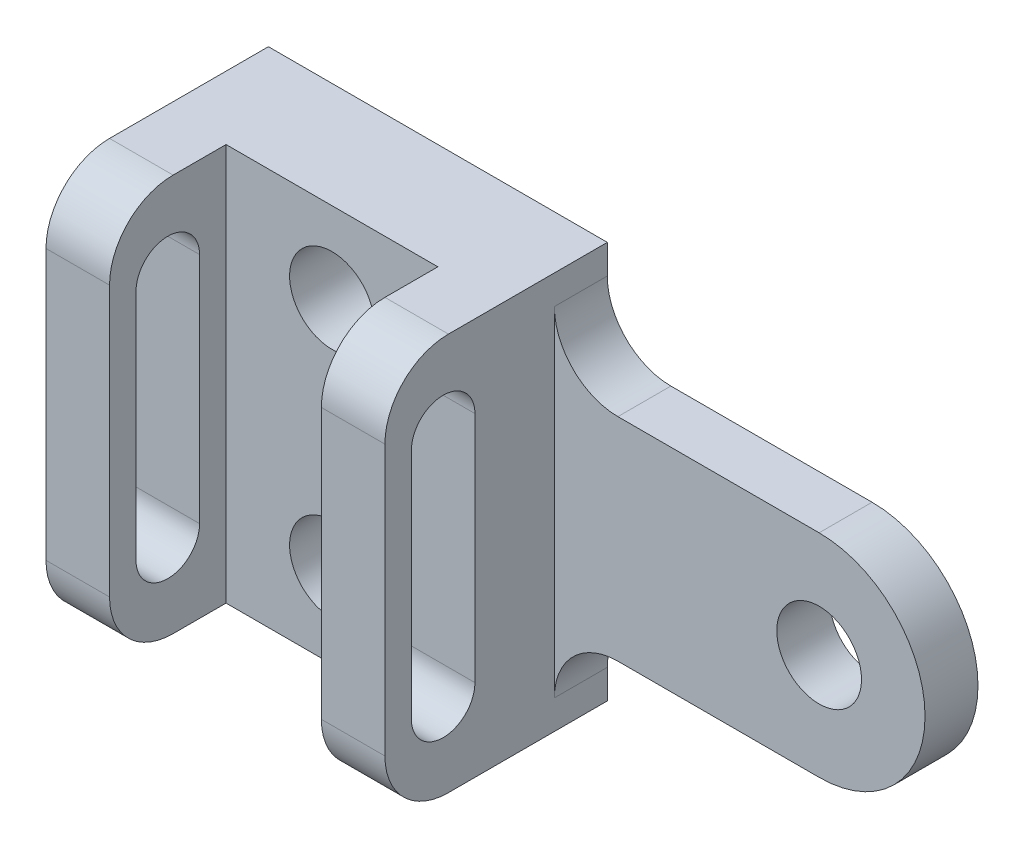
ISO-10303-21;
HEADER;
FILE_DESCRIPTION(('STEP AP214'),'2;1');
FILE_NAME('part.step','',(''),(''),'','','');
FILE_SCHEMA(('AUTOMOTIVE_DESIGN { 1 0 10303 214 1 1 1 1 }'));
ENDSEC;
DATA;
#1=APPLICATION_CONTEXT('core data for automotive mechanical design processes');
#2=APPLICATION_PROTOCOL_DEFINITION('international standard','automotive_design',2000,#1);
#3=PRODUCT_CONTEXT('',#1,'mechanical');
#4=PRODUCT('Part','Part','',(#3));
#5=PRODUCT_RELATED_PRODUCT_CATEGORY('part','',(#4));
#6=PRODUCT_DEFINITION_FORMATION('','',#4);
#7=PRODUCT_DEFINITION_CONTEXT('part definition',#1,'design');
#8=PRODUCT_DEFINITION('design','',#6,#7);
#9=PRODUCT_DEFINITION_SHAPE('','',#8);
#10=(LENGTH_UNIT() NAMED_UNIT(*) SI_UNIT(.MILLI.,.METRE.));
#11=(NAMED_UNIT(*) PLANE_ANGLE_UNIT() SI_UNIT($,.RADIAN.));
#12=(NAMED_UNIT(*) SI_UNIT($,.STERADIAN.) SOLID_ANGLE_UNIT());
#13=UNCERTAINTY_MEASURE_WITH_UNIT(LENGTH_MEASURE(1.E-05),#10,'distance_accuracy_value','');
#14=(GEOMETRIC_REPRESENTATION_CONTEXT(3) GLOBAL_UNCERTAINTY_ASSIGNED_CONTEXT((#13)) GLOBAL_UNIT_ASSIGNED_CONTEXT((#10,
#11,#12)) REPRESENTATION_CONTEXT('',''));
#15=CARTESIAN_POINT('',(0.,0.,0.));
#16=DIRECTION('',(0.,0.,1.));
#17=DIRECTION('',(1.,0.,0.));
#18=AXIS2_PLACEMENT_3D('',#15,#16,#17);
#19=CARTESIAN_POINT('',(0.,0.,20.));
#20=DIRECTION('',(0.,0.,1.));
#21=DIRECTION('',(1.,0.,0.));
#22=AXIS2_PLACEMENT_3D('',#19,#20,#21);
#23=PLANE('',#22);
#24=CARTESIAN_POINT('',(32.,59.5,20.));
#25=DIRECTION('',(0.,0.,1.));
#26=DIRECTION('',(1.,0.,0.));
#27=AXIS2_PLACEMENT_3D('',#24,#25,#26);
#28=CIRCLE('',#27,8.);
#29=CARTESIAN_POINT('',(40.,59.5,20.));
#30=VERTEX_POINT('',#29);
#31=EDGE_CURVE('E454',#30,#30,#28,.T.);
#32=ORIENTED_EDGE('',*,*,#31,.F.);
#33=EDGE_LOOP('',(#32));
#34=FACE_BOUND('',#33,.T.);
#35=CARTESIAN_POINT('',(32.,15.5,20.));
#36=DIRECTION('',(0.,0.,1.));
#37=DIRECTION('',(1.,0.,0.));
#38=AXIS2_PLACEMENT_3D('',#35,#36,#37);
#39=CIRCLE('',#38,8.);
#40=CARTESIAN_POINT('',(40.,15.5,20.));
#41=VERTEX_POINT('',#40);
#42=EDGE_CURVE('E450',#41,#41,#39,.T.);
#43=ORIENTED_EDGE('',*,*,#42,.F.);
#44=EDGE_LOOP('',(#43));
#45=FACE_BOUND('',#44,.T.);
#46=DIRECTION('',(1.,0.,0.));
#47=VECTOR('',#46,1.);
#48=CARTESIAN_POINT('',(0.,0.,20.));
#49=LINE('',#48,#47);
#50=CARTESIAN_POINT('',(12.,0.,20.));
#51=VERTEX_POINT('',#50);
#52=CARTESIAN_POINT('',(52.,0.,20.));
#53=VERTEX_POINT('',#52);
#54=EDGE_CURVE('E334',#51,#53,#49,.T.);
#55=ORIENTED_EDGE('',*,*,#54,.T.);
#56=DIRECTION('',(0.,-1.,0.));
#57=VECTOR('',#56,1.);
#58=CARTESIAN_POINT('',(52.,75.,20.));
#59=LINE('',#58,#57);
#60=CARTESIAN_POINT('',(52.,75.,20.));
#61=VERTEX_POINT('',#60);
#62=EDGE_CURVE('E305',#61,#53,#59,.T.);
#63=ORIENTED_EDGE('',*,*,#62,.F.);
#64=DIRECTION('',(-1.,0.,0.));
#65=VECTOR('',#64,1.);
#66=CARTESIAN_POINT('',(64.,75.,20.));
#67=LINE('',#66,#65);
#68=CARTESIAN_POINT('',(12.,75.,20.));
#69=VERTEX_POINT('',#68);
#70=EDGE_CURVE('E336',#61,#69,#67,.T.);
#71=ORIENTED_EDGE('',*,*,#70,.T.);
#72=DIRECTION('',(0.,1.,0.));
#73=VECTOR('',#72,1.);
#74=CARTESIAN_POINT('',(12.,75.,20.));
#75=LINE('',#74,#73);
#76=EDGE_CURVE('E322',#51,#69,#75,.T.);
#77=ORIENTED_EDGE('',*,*,#76,.F.);
#78=EDGE_LOOP('',(#55,#63,#71,#77));
#79=FACE_BOUND('',#78,.T.);
#80=ADVANCED_FACE('F39',(#34,#45,#79),#23,.T.);
#81=CARTESIAN_POINT('',(0.,75.,20.));
#82=DIRECTION('',(1.,0.,0.));
#83=DIRECTION('',(0.,0.,-1.));
#84=AXIS2_PLACEMENT_3D('',#81,#82,#83);
#85=PLANE('',#84);
#86=DIRECTION('',(0.,-1.,0.));
#87=VECTOR('',#86,1.);
#88=CARTESIAN_POINT('',(0.,15.5,37.));
#89=LINE('',#88,#87);
#90=CARTESIAN_POINT('',(0.,59.5,37.));
#91=VERTEX_POINT('',#90);
#92=CARTESIAN_POINT('',(0.,15.5,37.));
#93=VERTEX_POINT('',#92);
#94=EDGE_CURVE('E290',#91,#93,#89,.T.);
#95=ORIENTED_EDGE('',*,*,#94,.T.);
#96=CARTESIAN_POINT('',(0.,15.5,31.));
#97=DIRECTION('',(1.,0.,0.));
#98=DIRECTION('',(0.,1.,0.));
#99=AXIS2_PLACEMENT_3D('',#96,#97,#98);
#100=CIRCLE('',#99,6.00000000000001);
#101=CARTESIAN_POINT('',(0.,15.5,25.));
#102=VERTEX_POINT('',#101);
#103=EDGE_CURVE('E280',#93,#102,#100,.T.);
#104=ORIENTED_EDGE('',*,*,#103,.T.);
#105=DIRECTION('',(0.,1.,0.));
#106=VECTOR('',#105,1.);
#107=CARTESIAN_POINT('',(0.,15.5,25.));
#108=LINE('',#107,#106);
#109=CARTESIAN_POINT('',(0.,59.5,25.));
#110=VERTEX_POINT('',#109);
#111=EDGE_CURVE('E278',#102,#110,#108,.T.);
#112=ORIENTED_EDGE('',*,*,#111,.T.);
#113=CARTESIAN_POINT('',(0.,59.5,31.));
#114=DIRECTION('',(1.,0.,0.));
#115=DIRECTION('',(0.,1.,0.));
#116=AXIS2_PLACEMENT_3D('',#113,#114,#115);
#117=CIRCLE('',#116,6.00000000000001);
#118=EDGE_CURVE('E283',#110,#91,#117,.T.);
#119=ORIENTED_EDGE('',*,*,#118,.T.);
#120=EDGE_LOOP('',(#95,#104,#112,#119));
#121=FACE_BOUND('',#120,.T.);
#122=DIRECTION('',(0.,0.,-1.));
#123=VECTOR('',#122,1.);
#124=CARTESIAN_POINT('',(0.,0.,20.));
#125=LINE('',#124,#123);
#126=CARTESIAN_POINT('',(0.,0.,30.));
#127=VERTEX_POINT('',#126);
#128=CARTESIAN_POINT('',(0.,0.,0.));
#129=VERTEX_POINT('',#128);
#130=EDGE_CURVE('E356',#127,#129,#125,.T.);
#131=ORIENTED_EDGE('',*,*,#130,.F.);
#132=CARTESIAN_POINT('',(0.,12.,30.));
#133=DIRECTION('',(1.,0.,0.));
#134=DIRECTION('',(0.,0.,-1.));
#135=AXIS2_PLACEMENT_3D('',#132,#133,#134);
#136=CIRCLE('',#135,12.);
#137=CARTESIAN_POINT('',(0.,12.,42.));
#138=VERTEX_POINT('',#137);
#139=EDGE_CURVE('E372',#127,#138,#136,.F.);
#140=ORIENTED_EDGE('',*,*,#139,.T.);
#141=DIRECTION('',(0.,-1.,0.));
#142=VECTOR('',#141,1.);
#143=CARTESIAN_POINT('',(0.,75.,42.));
#144=LINE('',#143,#142);
#145=CARTESIAN_POINT('',(0.,63.,42.));
#146=VERTEX_POINT('',#145);
#147=EDGE_CURVE('E325',#146,#138,#144,.T.);
#148=ORIENTED_EDGE('',*,*,#147,.F.);
#149=CARTESIAN_POINT('',(0.,63.,30.));
#150=DIRECTION('',(1.,0.,0.));
#151=DIRECTION('',(0.,0.,-1.));
#152=AXIS2_PLACEMENT_3D('',#149,#150,#151);
#153=CIRCLE('',#152,12.);
#154=CARTESIAN_POINT('',(0.,75.,30.));
#155=VERTEX_POINT('',#154);
#156=EDGE_CURVE('E375',#146,#155,#153,.F.);
#157=ORIENTED_EDGE('',*,*,#156,.T.);
#158=DIRECTION('',(0.,0.,-1.));
#159=VECTOR('',#158,1.);
#160=CARTESIAN_POINT('',(0.,75.,20.));
#161=LINE('',#160,#159);
#162=CARTESIAN_POINT('',(0.,75.,0.));
#163=VERTEX_POINT('',#162);
#164=EDGE_CURVE('E345',#155,#163,#161,.T.);
#165=ORIENTED_EDGE('',*,*,#164,.T.);
#166=DIRECTION('',(0.,-1.,0.));
#167=VECTOR('',#166,1.);
#168=CARTESIAN_POINT('',(0.,75.,0.));
#169=LINE('',#168,#167);
#170=EDGE_CURVE('E332',#163,#129,#169,.T.);
#171=ORIENTED_EDGE('',*,*,#170,.T.);
#172=EDGE_LOOP('',(#131,#140,#148,#157,#165,#171));
#173=FACE_BOUND('',#172,.T.);
#174=ADVANCED_FACE('F472',(#121,#173),#85,.F.);
#175=CARTESIAN_POINT('',(0.,0.,20.));
#176=DIRECTION('',(0.,1.,0.));
#177=DIRECTION('',(0.,0.,1.));
#178=AXIS2_PLACEMENT_3D('',#175,#176,#177);
#179=PLANE('',#178);
#180=DIRECTION('',(0.,0.,-1.));
#181=VECTOR('',#180,1.);
#182=CARTESIAN_POINT('',(64.,0.,20.));
#183=LINE('',#182,#181);
#184=CARTESIAN_POINT('',(64.,0.,30.));
#185=VERTEX_POINT('',#184);
#186=CARTESIAN_POINT('',(64.,0.,0.));
#187=VERTEX_POINT('',#186);
#188=EDGE_CURVE('E358',#185,#187,#183,.T.);
#189=ORIENTED_EDGE('',*,*,#188,.F.);
#190=DIRECTION('',(1.,0.,0.));
#191=VECTOR('',#190,1.);
#192=CARTESIAN_POINT('',(52.,0.,30.));
#193=LINE('',#192,#191);
#194=CARTESIAN_POINT('',(52.,0.,30.));
#195=VERTEX_POINT('',#194);
#196=EDGE_CURVE('E65',#185,#195,#193,.F.);
#197=ORIENTED_EDGE('',*,*,#196,.T.);
#198=DIRECTION('',(0.,0.,-1.));
#199=VECTOR('',#198,1.);
#200=CARTESIAN_POINT('',(52.,0.,42.));
#201=LINE('',#200,#199);
#202=EDGE_CURVE('E316',#195,#53,#201,.T.);
#203=ORIENTED_EDGE('',*,*,#202,.T.);
#204=ORIENTED_EDGE('',*,*,#54,.F.);
#205=DIRECTION('',(0.,0.,-1.));
#206=VECTOR('',#205,1.);
#207=CARTESIAN_POINT('',(12.,0.,42.));
#208=LINE('',#207,#206);
#209=CARTESIAN_POINT('',(12.,0.,30.));
#210=VERTEX_POINT('',#209);
#211=EDGE_CURVE('E335',#210,#51,#208,.T.);
#212=ORIENTED_EDGE('',*,*,#211,.F.);
#213=DIRECTION('',(1.,0.,0.));
#214=VECTOR('',#213,1.);
#215=CARTESIAN_POINT('',(0.,0.,30.));
#216=LINE('',#215,#214);
#217=EDGE_CURVE('E369',#210,#127,#216,.F.);
#218=ORIENTED_EDGE('',*,*,#217,.T.);
#219=ORIENTED_EDGE('',*,*,#130,.T.);
#220=DIRECTION('',(1.,0.,0.));
#221=VECTOR('',#220,1.);
#222=CARTESIAN_POINT('',(0.,0.,0.));
#223=LINE('',#222,#221);
#224=EDGE_CURVE('E343',#129,#187,#223,.T.);
#225=ORIENTED_EDGE('',*,*,#224,.T.);
#226=EDGE_LOOP('',(#189,#197,#203,#204,#212,#218,#219,#225));
#227=FACE_BOUND('',#226,.T.);
#228=ADVANCED_FACE('F399',(#227),#179,.F.);
#229=CARTESIAN_POINT('',(64.,0.,20.));
#230=DIRECTION('',(-1.,0.,0.));
#231=DIRECTION('',(0.,0.,1.));
#232=AXIS2_PLACEMENT_3D('',#229,#230,#231);
#233=PLANE('',#232);
#234=DIRECTION('',(0.,-1.,0.));
#235=VECTOR('',#234,1.);
#236=CARTESIAN_POINT('',(64.,15.5,25.));
#237=LINE('',#236,#235);
#238=CARTESIAN_POINT('',(64.,59.5,25.));
#239=VERTEX_POINT('',#238);
#240=CARTESIAN_POINT('',(64.,15.5,25.));
#241=VERTEX_POINT('',#240);
#242=EDGE_CURVE('E260',#239,#241,#237,.T.);
#243=ORIENTED_EDGE('',*,*,#242,.T.);
#244=CARTESIAN_POINT('',(64.,15.5,31.));
#245=DIRECTION('',(-1.,0.,0.));
#246=DIRECTION('',(0.,-1.,0.));
#247=AXIS2_PLACEMENT_3D('',#244,#245,#246);
#248=CIRCLE('',#247,6.);
#249=CARTESIAN_POINT('',(64.,15.5,37.));
#250=VERTEX_POINT('',#249);
#251=EDGE_CURVE('E250',#241,#250,#248,.T.);
#252=ORIENTED_EDGE('',*,*,#251,.T.);
#253=DIRECTION('',(0.,1.,0.));
#254=VECTOR('',#253,1.);
#255=CARTESIAN_POINT('',(64.,15.5,37.));
#256=LINE('',#255,#254);
#257=CARTESIAN_POINT('',(64.,59.5,37.));
#258=VERTEX_POINT('',#257);
#259=EDGE_CURVE('E249',#250,#258,#256,.T.);
#260=ORIENTED_EDGE('',*,*,#259,.T.);
#261=CARTESIAN_POINT('',(64.,59.5,31.));
#262=DIRECTION('',(-1.,0.,0.));
#263=DIRECTION('',(0.,-1.,0.));
#264=AXIS2_PLACEMENT_3D('',#261,#262,#263);
#265=CIRCLE('',#264,6.);
#266=EDGE_CURVE('E251',#258,#239,#265,.T.);
#267=ORIENTED_EDGE('',*,*,#266,.T.);
#268=EDGE_LOOP('',(#243,#252,#260,#267));
#269=FACE_BOUND('',#268,.T.);
#270=DIRECTION('',(0.,1.,0.));
#271=VECTOR('',#270,1.);
#272=CARTESIAN_POINT('',(64.,75.,42.));
#273=LINE('',#272,#271);
#274=CARTESIAN_POINT('',(64.,12.,42.));
#275=VERTEX_POINT('',#274);
#276=CARTESIAN_POINT('',(64.,63.,42.));
#277=VERTEX_POINT('',#276);
#278=EDGE_CURVE('E315',#275,#277,#273,.T.);
#279=ORIENTED_EDGE('',*,*,#278,.F.);
#280=CARTESIAN_POINT('',(64.,12.,30.));
#281=DIRECTION('',(-1.,0.,0.));
#282=DIRECTION('',(0.,0.,1.));
#283=AXIS2_PLACEMENT_3D('',#280,#281,#282);
#284=CIRCLE('',#283,12.);
#285=EDGE_CURVE('E387',#275,#185,#284,.F.);
#286=ORIENTED_EDGE('',*,*,#285,.T.);
#287=ORIENTED_EDGE('',*,*,#188,.T.);
#288=DIRECTION('',(0.,1.,0.));
#289=VECTOR('',#288,1.);
#290=CARTESIAN_POINT('',(64.,0.,0.));
#291=LINE('',#290,#289);
#292=CARTESIAN_POINT('',(64.,5.49999999999997,0.));
#293=VERTEX_POINT('',#292);
#294=EDGE_CURVE('E348',#187,#293,#291,.T.);
#295=ORIENTED_EDGE('',*,*,#294,.T.);
#296=DIRECTION('',(0.,0.,-1.));
#297=VECTOR('',#296,1.);
#298=CARTESIAN_POINT('',(64.,5.49999999999997,10.));
#299=LINE('',#298,#297);
#300=CARTESIAN_POINT('',(64.,5.49999999999997,10.));
#301=VERTEX_POINT('',#300);
#302=EDGE_CURVE('E411',#301,#293,#299,.T.);
#303=ORIENTED_EDGE('',*,*,#302,.F.);
#304=DIRECTION('',(0.,-1.,0.));
#305=VECTOR('',#304,1.);
#306=CARTESIAN_POINT('',(64.,69.5,10.));
#307=LINE('',#306,#305);
#308=CARTESIAN_POINT('',(64.,69.5,10.));
#309=VERTEX_POINT('',#308);
#310=EDGE_CURVE('E438',#309,#301,#307,.T.);
#311=ORIENTED_EDGE('',*,*,#310,.F.);
#312=DIRECTION('',(0.,0.,-1.));
#313=VECTOR('',#312,1.);
#314=CARTESIAN_POINT('',(64.,69.5,10.));
#315=LINE('',#314,#313);
#316=CARTESIAN_POINT('',(64.,69.5,0.));
#317=VERTEX_POINT('',#316);
#318=EDGE_CURVE('E243',#309,#317,#315,.T.);
#319=ORIENTED_EDGE('',*,*,#318,.T.);
#320=CARTESIAN_POINT('',(64.,75.,0.));
#321=VERTEX_POINT('',#320);
#322=EDGE_CURVE('E350',#317,#321,#291,.T.);
#323=ORIENTED_EDGE('',*,*,#322,.T.);
#324=DIRECTION('',(0.,0.,-1.));
#325=VECTOR('',#324,1.);
#326=CARTESIAN_POINT('',(64.,75.,20.));
#327=LINE('',#326,#325);
#328=CARTESIAN_POINT('',(64.,75.,30.));
#329=VERTEX_POINT('',#328);
#330=EDGE_CURVE('E352',#329,#321,#327,.T.);
#331=ORIENTED_EDGE('',*,*,#330,.F.);
#332=CARTESIAN_POINT('',(64.,63.,30.));
#333=DIRECTION('',(-1.,0.,0.));
#334=DIRECTION('',(0.,0.,1.));
#335=AXIS2_PLACEMENT_3D('',#332,#333,#334);
#336=CIRCLE('',#335,12.);
#337=EDGE_CURVE('E381',#329,#277,#336,.F.);
#338=ORIENTED_EDGE('',*,*,#337,.T.);
#339=EDGE_LOOP('',(#279,#286,#287,#295,#303,#311,#319,#323,#331,#338));
#340=FACE_BOUND('',#339,.T.);
#341=ADVANCED_FACE('F397',(#269,#340),#233,.F.);
#342=CARTESIAN_POINT('',(64.,75.,20.));
#343=DIRECTION('',(0.,-1.,0.));
#344=DIRECTION('',(0.,0.,-1.));
#345=AXIS2_PLACEMENT_3D('',#342,#343,#344);
#346=PLANE('',#345);
#347=DIRECTION('',(0.,0.,-1.));
#348=VECTOR('',#347,1.);
#349=CARTESIAN_POINT('',(52.,75.,42.));
#350=LINE('',#349,#348);
#351=CARTESIAN_POINT('',(52.,75.,30.));
#352=VERTEX_POINT('',#351);
#353=EDGE_CURVE('E314',#352,#61,#350,.T.);
#354=ORIENTED_EDGE('',*,*,#353,.F.);
#355=DIRECTION('',(-1.,0.,0.));
#356=VECTOR('',#355,1.);
#357=CARTESIAN_POINT('',(64.,75.,30.));
#358=LINE('',#357,#356);
#359=EDGE_CURVE('E11',#352,#329,#358,.F.);
#360=ORIENTED_EDGE('',*,*,#359,.T.);
#361=ORIENTED_EDGE('',*,*,#330,.T.);
#362=DIRECTION('',(-1.,0.,0.));
#363=VECTOR('',#362,1.);
#364=CARTESIAN_POINT('',(64.,75.,0.));
#365=LINE('',#364,#363);
#366=EDGE_CURVE('E339',#321,#163,#365,.T.);
#367=ORIENTED_EDGE('',*,*,#366,.T.);
#368=ORIENTED_EDGE('',*,*,#164,.F.);
#369=DIRECTION('',(-1.,0.,0.));
#370=VECTOR('',#369,1.);
#371=CARTESIAN_POINT('',(12.,75.,30.));
#372=LINE('',#371,#370);
#373=CARTESIAN_POINT('',(12.,75.,30.));
#374=VERTEX_POINT('',#373);
#375=EDGE_CURVE('E376',#155,#374,#372,.F.);
#376=ORIENTED_EDGE('',*,*,#375,.T.);
#377=DIRECTION('',(0.,0.,-1.));
#378=VECTOR('',#377,1.);
#379=CARTESIAN_POINT('',(12.,75.,42.));
#380=LINE('',#379,#378);
#381=EDGE_CURVE('E330',#374,#69,#380,.T.);
#382=ORIENTED_EDGE('',*,*,#381,.T.);
#383=ORIENTED_EDGE('',*,*,#70,.F.);
#384=EDGE_LOOP('',(#354,#360,#361,#367,#368,#376,#382,#383));
#385=FACE_BOUND('',#384,.T.);
#386=ADVANCED_FACE('F485',(#385),#346,.F.);
#387=CARTESIAN_POINT('',(0.,0.,0.));
#388=DIRECTION('',(0.,0.,1.));
#389=DIRECTION('',(1.,0.,0.));
#390=AXIS2_PLACEMENT_3D('',#387,#388,#389);
#391=PLANE('',#390);
#392=CARTESIAN_POINT('',(32.,59.5,0.));
#393=DIRECTION('',(0.,0.,1.));
#394=DIRECTION('',(1.,0.,0.));
#395=AXIS2_PLACEMENT_3D('',#392,#393,#394);
#396=CIRCLE('',#395,8.);
#397=CARTESIAN_POINT('',(40.,59.5,0.));
#398=VERTEX_POINT('',#397);
#399=EDGE_CURVE('E443',#398,#398,#396,.T.);
#400=ORIENTED_EDGE('',*,*,#399,.T.);
#401=EDGE_LOOP('',(#400));
#402=FACE_BOUND('',#401,.T.);
#403=CARTESIAN_POINT('',(32.,15.5,0.));
#404=DIRECTION('',(0.,0.,1.));
#405=DIRECTION('',(1.,0.,0.));
#406=AXIS2_PLACEMENT_3D('',#403,#404,#405);
#407=CIRCLE('',#406,8.);
#408=CARTESIAN_POINT('',(40.,15.5,0.));
#409=VERTEX_POINT('',#408);
#410=EDGE_CURVE('E448',#409,#409,#407,.T.);
#411=ORIENTED_EDGE('',*,*,#410,.T.);
#412=EDGE_LOOP('',(#411));
#413=FACE_BOUND('',#412,.T.);
#414=ORIENTED_EDGE('',*,*,#170,.F.);
#415=ORIENTED_EDGE('',*,*,#366,.F.);
#416=ORIENTED_EDGE('',*,*,#322,.F.);
#417=CARTESIAN_POINT('',(76.,69.5,0.));
#418=DIRECTION('',(0.,0.,-1.));
#419=DIRECTION('',(1.,0.,0.));
#420=AXIS2_PLACEMENT_3D('',#417,#418,#419);
#421=CIRCLE('',#420,12.);
#422=CARTESIAN_POINT('',(76.,57.5,0.));
#423=VERTEX_POINT('',#422);
#424=EDGE_CURVE('E429',#423,#317,#421,.T.);
#425=ORIENTED_EDGE('',*,*,#424,.F.);
#426=DIRECTION('',(-1.,0.,0.));
#427=VECTOR('',#426,1.);
#428=CARTESIAN_POINT('',(114.,57.5,0.));
#429=LINE('',#428,#427);
#430=CARTESIAN_POINT('',(114.,57.5,0.));
#431=VERTEX_POINT('',#430);
#432=EDGE_CURVE('E435',#431,#423,#429,.T.);
#433=ORIENTED_EDGE('',*,*,#432,.F.);
#434=CARTESIAN_POINT('',(114.,37.5,0.));
#435=DIRECTION('',(0.,0.,1.));
#436=DIRECTION('',(1.,0.,0.));
#437=AXIS2_PLACEMENT_3D('',#434,#435,#436);
#438=CIRCLE('',#437,20.);
#439=CARTESIAN_POINT('',(114.,17.5,0.));
#440=VERTEX_POINT('',#439);
#441=EDGE_CURVE('E238',#440,#431,#438,.T.);
#442=ORIENTED_EDGE('',*,*,#441,.F.);
#443=DIRECTION('',(1.,0.,0.));
#444=VECTOR('',#443,1.);
#445=CARTESIAN_POINT('',(114.,17.5,0.));
#446=LINE('',#445,#444);
#447=CARTESIAN_POINT('',(76.,17.5,0.));
#448=VERTEX_POINT('',#447);
#449=EDGE_CURVE('E234',#448,#440,#446,.T.);
#450=ORIENTED_EDGE('',*,*,#449,.F.);
#451=CARTESIAN_POINT('',(76.,5.49999999999997,0.));
#452=DIRECTION('',(0.,0.,-1.));
#453=DIRECTION('',(1.,0.,0.));
#454=AXIS2_PLACEMENT_3D('',#451,#452,#453);
#455=CIRCLE('',#454,12.);
#456=EDGE_CURVE('E408',#293,#448,#455,.T.);
#457=ORIENTED_EDGE('',*,*,#456,.F.);
#458=ORIENTED_EDGE('',*,*,#294,.F.);
#459=ORIENTED_EDGE('',*,*,#224,.F.);
#460=EDGE_LOOP('',(#414,#415,#416,#425,#433,#442,#450,#457,#458,#459));
#461=FACE_BOUND('',#460,.T.);
#462=CARTESIAN_POINT('',(114.,37.5,0.));
#463=DIRECTION('',(0.,0.,1.));
#464=DIRECTION('',(1.,0.,0.));
#465=AXIS2_PLACEMENT_3D('',#462,#463,#464);
#466=CIRCLE('',#465,8.);
#467=CARTESIAN_POINT('',(122.,37.5,0.));
#468=VERTEX_POINT('',#467);
#469=EDGE_CURVE('E441',#468,#468,#466,.T.);
#470=ORIENTED_EDGE('',*,*,#469,.T.);
#471=EDGE_LOOP('',(#470));
#472=FACE_BOUND('',#471,.T.);
#473=ADVANCED_FACE('F410',(#402,#413,#461,#472),#391,.F.);
#474=CARTESIAN_POINT('',(12.,75.,42.));
#475=DIRECTION('',(-1.,0.,0.));
#476=DIRECTION('',(0.,-1.,0.));
#477=AXIS2_PLACEMENT_3D('',#474,#475,#476);
#478=PLANE('',#477);
#479=DIRECTION('',(0.,1.,0.));
#480=VECTOR('',#479,1.);
#481=CARTESIAN_POINT('',(12.,15.5,25.));
#482=LINE('',#481,#480);
#483=CARTESIAN_POINT('',(12.,15.5,25.));
#484=VERTEX_POINT('',#483);
#485=CARTESIAN_POINT('',(12.,59.5,25.));
#486=VERTEX_POINT('',#485);
#487=EDGE_CURVE('E292',#484,#486,#482,.T.);
#488=ORIENTED_EDGE('',*,*,#487,.F.);
#489=CARTESIAN_POINT('',(12.,15.5,31.));
#490=DIRECTION('',(1.,0.,0.));
#491=DIRECTION('',(0.,1.,0.));
#492=AXIS2_PLACEMENT_3D('',#489,#490,#491);
#493=CIRCLE('',#492,6.00000000000001);
#494=CARTESIAN_POINT('',(12.,15.5,37.));
#495=VERTEX_POINT('',#494);
#496=EDGE_CURVE('E269',#495,#484,#493,.T.);
#497=ORIENTED_EDGE('',*,*,#496,.F.);
#498=DIRECTION('',(0.,-1.,0.));
#499=VECTOR('',#498,1.);
#500=CARTESIAN_POINT('',(12.,15.5,37.));
#501=LINE('',#500,#499);
#502=CARTESIAN_POINT('',(12.,59.5,37.));
#503=VERTEX_POINT('',#502);
#504=EDGE_CURVE('E284',#503,#495,#501,.T.);
#505=ORIENTED_EDGE('',*,*,#504,.F.);
#506=CARTESIAN_POINT('',(12.,59.5,31.));
#507=DIRECTION('',(1.,0.,0.));
#508=DIRECTION('',(0.,1.,0.));
#509=AXIS2_PLACEMENT_3D('',#506,#507,#508);
#510=CIRCLE('',#509,6.00000000000001);
#511=EDGE_CURVE('E294',#486,#503,#510,.T.);
#512=ORIENTED_EDGE('',*,*,#511,.F.);
#513=EDGE_LOOP('',(#488,#497,#505,#512));
#514=FACE_BOUND('',#513,.T.);
#515=DIRECTION('',(0.,1.,0.));
#516=VECTOR('',#515,1.);
#517=CARTESIAN_POINT('',(12.,75.,42.));
#518=LINE('',#517,#516);
#519=CARTESIAN_POINT('',(12.,12.,42.));
#520=VERTEX_POINT('',#519);
#521=CARTESIAN_POINT('',(12.,63.,42.));
#522=VERTEX_POINT('',#521);
#523=EDGE_CURVE('E323',#520,#522,#518,.T.);
#524=ORIENTED_EDGE('',*,*,#523,.F.);
#525=CARTESIAN_POINT('',(12.,12.,30.));
#526=DIRECTION('',(-1.,0.,0.));
#527=DIRECTION('',(0.,-1.,0.));
#528=AXIS2_PLACEMENT_3D('',#525,#526,#527);
#529=CIRCLE('',#528,12.);
#530=EDGE_CURVE('E368',#520,#210,#529,.F.);
#531=ORIENTED_EDGE('',*,*,#530,.T.);
#532=ORIENTED_EDGE('',*,*,#211,.T.);
#533=ORIENTED_EDGE('',*,*,#76,.T.);
#534=ORIENTED_EDGE('',*,*,#381,.F.);
#535=CARTESIAN_POINT('',(12.,63.,30.));
#536=DIRECTION('',(-1.,0.,0.));
#537=DIRECTION('',(0.,-1.,0.));
#538=AXIS2_PLACEMENT_3D('',#535,#536,#537);
#539=CIRCLE('',#538,12.);
#540=EDGE_CURVE('E366',#374,#522,#539,.F.);
#541=ORIENTED_EDGE('',*,*,#540,.T.);
#542=EDGE_LOOP('',(#524,#531,#532,#533,#534,#541));
#543=FACE_BOUND('',#542,.T.);
#544=ADVANCED_FACE('F488',(#514,#543),#478,.F.);
#545=CARTESIAN_POINT('',(0.,0.,42.));
#546=DIRECTION('',(0.,0.,1.));
#547=DIRECTION('',(1.,0.,0.));
#548=AXIS2_PLACEMENT_3D('',#545,#546,#547);
#549=PLANE('',#548);
#550=ORIENTED_EDGE('',*,*,#147,.T.);
#551=DIRECTION('',(1.,0.,0.));
#552=VECTOR('',#551,1.);
#553=CARTESIAN_POINT('',(12.,12.,42.));
#554=LINE('',#553,#552);
#555=EDGE_CURVE('E361',#138,#520,#554,.T.);
#556=ORIENTED_EDGE('',*,*,#555,.T.);
#557=ORIENTED_EDGE('',*,*,#523,.T.);
#558=DIRECTION('',(-1.,0.,0.));
#559=VECTOR('',#558,1.);
#560=CARTESIAN_POINT('',(0.,63.,42.));
#561=LINE('',#560,#559);
#562=EDGE_CURVE('E359',#522,#146,#561,.T.);
#563=ORIENTED_EDGE('',*,*,#562,.T.);
#564=EDGE_LOOP('',(#550,#556,#557,#563));
#565=FACE_BOUND('',#564,.T.);
#566=ADVANCED_FACE('F492',(#565),#549,.T.);
#567=CARTESIAN_POINT('',(52.,75.,42.));
#568=DIRECTION('',(1.,0.,0.));
#569=DIRECTION('',(0.,1.,0.));
#570=AXIS2_PLACEMENT_3D('',#567,#568,#569);
#571=PLANE('',#570);
#572=DIRECTION('',(0.,1.,0.));
#573=VECTOR('',#572,1.);
#574=CARTESIAN_POINT('',(52.,15.5,37.));
#575=LINE('',#574,#573);
#576=CARTESIAN_POINT('',(52.,15.5,37.));
#577=VERTEX_POINT('',#576);
#578=CARTESIAN_POINT('',(52.,59.5,37.));
#579=VERTEX_POINT('',#578);
#580=EDGE_CURVE('E241',#577,#579,#575,.T.);
#581=ORIENTED_EDGE('',*,*,#580,.F.);
#582=CARTESIAN_POINT('',(52.,15.5,31.));
#583=DIRECTION('',(-1.,0.,0.));
#584=DIRECTION('',(0.,-1.,0.));
#585=AXIS2_PLACEMENT_3D('',#582,#583,#584);
#586=CIRCLE('',#585,6.);
#587=CARTESIAN_POINT('',(52.,15.5,25.));
#588=VERTEX_POINT('',#587);
#589=EDGE_CURVE('E237',#588,#577,#586,.T.);
#590=ORIENTED_EDGE('',*,*,#589,.F.);
#591=DIRECTION('',(0.,-1.,0.));
#592=VECTOR('',#591,1.);
#593=CARTESIAN_POINT('',(52.,15.5,25.));
#594=LINE('',#593,#592);
#595=CARTESIAN_POINT('',(52.,59.5,25.));
#596=VERTEX_POINT('',#595);
#597=EDGE_CURVE('E252',#596,#588,#594,.T.);
#598=ORIENTED_EDGE('',*,*,#597,.F.);
#599=CARTESIAN_POINT('',(52.,59.5,31.));
#600=DIRECTION('',(-1.,0.,0.));
#601=DIRECTION('',(0.,-1.,0.));
#602=AXIS2_PLACEMENT_3D('',#599,#600,#601);
#603=CIRCLE('',#602,6.);
#604=EDGE_CURVE('E265',#579,#596,#603,.T.);
#605=ORIENTED_EDGE('',*,*,#604,.F.);
#606=EDGE_LOOP('',(#581,#590,#598,#605));
#607=FACE_BOUND('',#606,.T.);
#608=ORIENTED_EDGE('',*,*,#202,.F.);
#609=CARTESIAN_POINT('',(52.,12.,30.));
#610=DIRECTION('',(1.,0.,0.));
#611=DIRECTION('',(0.,1.,0.));
#612=AXIS2_PLACEMENT_3D('',#609,#610,#611);
#613=CIRCLE('',#612,12.);
#614=CARTESIAN_POINT('',(52.,12.,42.));
#615=VERTEX_POINT('',#614);
#616=EDGE_CURVE('E50',#195,#615,#613,.F.);
#617=ORIENTED_EDGE('',*,*,#616,.T.);
#618=DIRECTION('',(0.,-1.,0.));
#619=VECTOR('',#618,1.);
#620=CARTESIAN_POINT('',(52.,75.,42.));
#621=LINE('',#620,#619);
#622=CARTESIAN_POINT('',(52.,63.,42.));
#623=VERTEX_POINT('',#622);
#624=EDGE_CURVE('E307',#623,#615,#621,.T.);
#625=ORIENTED_EDGE('',*,*,#624,.F.);
#626=CARTESIAN_POINT('',(52.,63.,30.));
#627=DIRECTION('',(1.,0.,0.));
#628=DIRECTION('',(0.,1.,0.));
#629=AXIS2_PLACEMENT_3D('',#626,#627,#628);
#630=CIRCLE('',#629,12.);
#631=EDGE_CURVE('E53',#623,#352,#630,.F.);
#632=ORIENTED_EDGE('',*,*,#631,.T.);
#633=ORIENTED_EDGE('',*,*,#353,.T.);
#634=ORIENTED_EDGE('',*,*,#62,.T.);
#635=EDGE_LOOP('',(#608,#617,#625,#632,#633,#634));
#636=FACE_BOUND('',#635,.T.);
#637=ADVANCED_FACE('F388',(#607,#636),#571,.F.);
#638=CARTESIAN_POINT('',(0.,0.,42.));
#639=DIRECTION('',(0.,0.,1.));
#640=DIRECTION('',(1.,0.,0.));
#641=AXIS2_PLACEMENT_3D('',#638,#639,#640);
#642=PLANE('',#641);
#643=ORIENTED_EDGE('',*,*,#624,.T.);
#644=DIRECTION('',(1.,0.,0.));
#645=VECTOR('',#644,1.);
#646=CARTESIAN_POINT('',(64.,12.,42.));
#647=LINE('',#646,#645);
#648=EDGE_CURVE('E382',#615,#275,#647,.T.);
#649=ORIENTED_EDGE('',*,*,#648,.T.);
#650=ORIENTED_EDGE('',*,*,#278,.T.);
#651=DIRECTION('',(-1.,0.,0.));
#652=VECTOR('',#651,1.);
#653=CARTESIAN_POINT('',(52.,63.,42.));
#654=LINE('',#653,#652);
#655=EDGE_CURVE('E377',#277,#623,#654,.T.);
#656=ORIENTED_EDGE('',*,*,#655,.T.);
#657=EDGE_LOOP('',(#643,#649,#650,#656));
#658=FACE_BOUND('',#657,.T.);
#659=ADVANCED_FACE('F393',(#658),#642,.T.);
#660=CARTESIAN_POINT('',(0.,15.5,31.));
#661=DIRECTION('',(1.,0.,0.));
#662=DIRECTION('',(0.,1.,0.));
#663=AXIS2_PLACEMENT_3D('',#660,#661,#662);
#664=CYLINDRICAL_SURFACE('',#663,6.00000000000001);
#665=ORIENTED_EDGE('',*,*,#496,.T.);
#666=DIRECTION('',(1.,0.,0.));
#667=VECTOR('',#666,1.);
#668=CARTESIAN_POINT('',(0.,15.5,25.));
#669=LINE('',#668,#667);
#670=EDGE_CURVE('E289',#102,#484,#669,.T.);
#671=ORIENTED_EDGE('',*,*,#670,.F.);
#672=ORIENTED_EDGE('',*,*,#103,.F.);
#673=DIRECTION('',(1.,0.,0.));
#674=VECTOR('',#673,1.);
#675=CARTESIAN_POINT('',(0.,15.5,37.));
#676=LINE('',#675,#674);
#677=EDGE_CURVE('E297',#93,#495,#676,.T.);
#678=ORIENTED_EDGE('',*,*,#677,.T.);
#679=EDGE_LOOP('',(#665,#671,#672,#678));
#680=FACE_BOUND('',#679,.T.);
#681=ADVANCED_FACE('F547',(#680),#664,.F.);
#682=CARTESIAN_POINT('',(0.,15.5,37.));
#683=DIRECTION('',(0.,0.,1.));
#684=DIRECTION('',(1.,0.,0.));
#685=AXIS2_PLACEMENT_3D('',#682,#683,#684);
#686=PLANE('',#685);
#687=ORIENTED_EDGE('',*,*,#504,.T.);
#688=ORIENTED_EDGE('',*,*,#677,.F.);
#689=ORIENTED_EDGE('',*,*,#94,.F.);
#690=DIRECTION('',(1.,0.,0.));
#691=VECTOR('',#690,1.);
#692=CARTESIAN_POINT('',(0.,59.5,37.));
#693=LINE('',#692,#691);
#694=EDGE_CURVE('E303',#91,#503,#693,.T.);
#695=ORIENTED_EDGE('',*,*,#694,.T.);
#696=EDGE_LOOP('',(#687,#688,#689,#695));
#697=FACE_BOUND('',#696,.T.);
#698=ADVANCED_FACE('F542',(#697),#686,.F.);
#699=CARTESIAN_POINT('',(0.,59.5,31.));
#700=DIRECTION('',(1.,0.,0.));
#701=DIRECTION('',(0.,1.,0.));
#702=AXIS2_PLACEMENT_3D('',#699,#700,#701);
#703=CYLINDRICAL_SURFACE('',#702,6.00000000000001);
#704=ORIENTED_EDGE('',*,*,#511,.T.);
#705=ORIENTED_EDGE('',*,*,#694,.F.);
#706=ORIENTED_EDGE('',*,*,#118,.F.);
#707=DIRECTION('',(1.,0.,0.));
#708=VECTOR('',#707,1.);
#709=CARTESIAN_POINT('',(0.,59.5,25.));
#710=LINE('',#709,#708);
#711=EDGE_CURVE('E304',#110,#486,#710,.T.);
#712=ORIENTED_EDGE('',*,*,#711,.T.);
#713=EDGE_LOOP('',(#704,#705,#706,#712));
#714=FACE_BOUND('',#713,.T.);
#715=ADVANCED_FACE('F548',(#714),#703,.F.);
#716=CARTESIAN_POINT('',(0.,15.5,25.));
#717=DIRECTION('',(0.,0.,-1.));
#718=DIRECTION('',(-1.,0.,0.));
#719=AXIS2_PLACEMENT_3D('',#716,#717,#718);
#720=PLANE('',#719);
#721=ORIENTED_EDGE('',*,*,#487,.T.);
#722=ORIENTED_EDGE('',*,*,#711,.F.);
#723=ORIENTED_EDGE('',*,*,#111,.F.);
#724=ORIENTED_EDGE('',*,*,#670,.T.);
#725=EDGE_LOOP('',(#721,#722,#723,#724));
#726=FACE_BOUND('',#725,.T.);
#727=ADVANCED_FACE('F545',(#726),#720,.F.);
#728=CARTESIAN_POINT('',(64.,15.5,31.));
#729=DIRECTION('',(-1.,0.,0.));
#730=DIRECTION('',(0.,-1.,0.));
#731=AXIS2_PLACEMENT_3D('',#728,#729,#730);
#732=CYLINDRICAL_SURFACE('',#731,6.);
#733=ORIENTED_EDGE('',*,*,#589,.T.);
#734=DIRECTION('',(-1.,0.,0.));
#735=VECTOR('',#734,1.);
#736=CARTESIAN_POINT('',(64.,15.5,37.));
#737=LINE('',#736,#735);
#738=EDGE_CURVE('E256',#250,#577,#737,.T.);
#739=ORIENTED_EDGE('',*,*,#738,.F.);
#740=ORIENTED_EDGE('',*,*,#251,.F.);
#741=DIRECTION('',(-1.,0.,0.));
#742=VECTOR('',#741,1.);
#743=CARTESIAN_POINT('',(64.,15.5,25.));
#744=LINE('',#743,#742);
#745=EDGE_CURVE('E268',#241,#588,#744,.T.);
#746=ORIENTED_EDGE('',*,*,#745,.T.);
#747=EDGE_LOOP('',(#733,#739,#740,#746));
#748=FACE_BOUND('',#747,.T.);
#749=ADVANCED_FACE('F535',(#748),#732,.F.);
#750=CARTESIAN_POINT('',(64.,15.5,25.));
#751=DIRECTION('',(0.,0.,-1.));
#752=DIRECTION('',(-1.,0.,0.));
#753=AXIS2_PLACEMENT_3D('',#750,#751,#752);
#754=PLANE('',#753);
#755=ORIENTED_EDGE('',*,*,#597,.T.);
#756=ORIENTED_EDGE('',*,*,#745,.F.);
#757=ORIENTED_EDGE('',*,*,#242,.F.);
#758=DIRECTION('',(-1.,0.,0.));
#759=VECTOR('',#758,1.);
#760=CARTESIAN_POINT('',(64.,59.5,25.));
#761=LINE('',#760,#759);
#762=EDGE_CURVE('E272',#239,#596,#761,.T.);
#763=ORIENTED_EDGE('',*,*,#762,.T.);
#764=EDGE_LOOP('',(#755,#756,#757,#763));
#765=FACE_BOUND('',#764,.T.);
#766=ADVANCED_FACE('F528',(#765),#754,.F.);
#767=CARTESIAN_POINT('',(64.,59.5,31.));
#768=DIRECTION('',(-1.,0.,0.));
#769=DIRECTION('',(0.,-1.,0.));
#770=AXIS2_PLACEMENT_3D('',#767,#768,#769);
#771=CYLINDRICAL_SURFACE('',#770,6.);
#772=ORIENTED_EDGE('',*,*,#604,.T.);
#773=ORIENTED_EDGE('',*,*,#762,.F.);
#774=ORIENTED_EDGE('',*,*,#266,.F.);
#775=DIRECTION('',(-1.,0.,0.));
#776=VECTOR('',#775,1.);
#777=CARTESIAN_POINT('',(64.,59.5,37.));
#778=LINE('',#777,#776);
#779=EDGE_CURVE('E271',#258,#579,#778,.T.);
#780=ORIENTED_EDGE('',*,*,#779,.T.);
#781=EDGE_LOOP('',(#772,#773,#774,#780));
#782=FACE_BOUND('',#781,.T.);
#783=ADVANCED_FACE('F532',(#782),#771,.F.);
#784=CARTESIAN_POINT('',(64.,15.5,37.));
#785=DIRECTION('',(0.,0.,1.));
#786=DIRECTION('',(1.,0.,0.));
#787=AXIS2_PLACEMENT_3D('',#784,#785,#786);
#788=PLANE('',#787);
#789=ORIENTED_EDGE('',*,*,#580,.T.);
#790=ORIENTED_EDGE('',*,*,#779,.F.);
#791=ORIENTED_EDGE('',*,*,#259,.F.);
#792=ORIENTED_EDGE('',*,*,#738,.T.);
#793=EDGE_LOOP('',(#789,#790,#791,#792));
#794=FACE_BOUND('',#793,.T.);
#795=ADVANCED_FACE('F537',(#794),#788,.F.);
#796=CARTESIAN_POINT('',(114.,37.5,10.));
#797=DIRECTION('',(0.,0.,1.));
#798=DIRECTION('',(1.,0.,0.));
#799=AXIS2_PLACEMENT_3D('',#796,#797,#798);
#800=PLANE('',#799);
#801=CARTESIAN_POINT('',(114.,37.5,10.));
#802=DIRECTION('',(0.,0.,1.));
#803=DIRECTION('',(1.,0.,0.));
#804=AXIS2_PLACEMENT_3D('',#801,#802,#803);
#805=CIRCLE('',#804,20.);
#806=CARTESIAN_POINT('',(114.,17.5,10.));
#807=VERTEX_POINT('',#806);
#808=CARTESIAN_POINT('',(114.,57.5,10.));
#809=VERTEX_POINT('',#808);
#810=EDGE_CURVE('E222',#807,#809,#805,.T.);
#811=ORIENTED_EDGE('',*,*,#810,.T.);
#812=DIRECTION('',(-1.,0.,0.));
#813=VECTOR('',#812,1.);
#814=CARTESIAN_POINT('',(114.,57.5,10.));
#815=LINE('',#814,#813);
#816=CARTESIAN_POINT('',(76.,57.5,10.));
#817=VERTEX_POINT('',#816);
#818=EDGE_CURVE('E215',#809,#817,#815,.T.);
#819=ORIENTED_EDGE('',*,*,#818,.T.);
#820=CARTESIAN_POINT('',(76.,69.5,10.));
#821=DIRECTION('',(0.,0.,-1.));
#822=DIRECTION('',(1.,0.,0.));
#823=AXIS2_PLACEMENT_3D('',#820,#821,#822);
#824=CIRCLE('',#823,12.);
#825=EDGE_CURVE('E223',#817,#309,#824,.T.);
#826=ORIENTED_EDGE('',*,*,#825,.T.);
#827=ORIENTED_EDGE('',*,*,#310,.T.);
#828=CARTESIAN_POINT('',(76.,5.49999999999997,10.));
#829=DIRECTION('',(0.,0.,-1.));
#830=DIRECTION('',(1.,0.,0.));
#831=AXIS2_PLACEMENT_3D('',#828,#829,#830);
#832=CIRCLE('',#831,12.);
#833=CARTESIAN_POINT('',(76.,17.5,10.));
#834=VERTEX_POINT('',#833);
#835=EDGE_CURVE('E417',#301,#834,#832,.T.);
#836=ORIENTED_EDGE('',*,*,#835,.T.);
#837=DIRECTION('',(1.,0.,0.));
#838=VECTOR('',#837,1.);
#839=CARTESIAN_POINT('',(114.,17.5,10.));
#840=LINE('',#839,#838);
#841=EDGE_CURVE('E229',#834,#807,#840,.T.);
#842=ORIENTED_EDGE('',*,*,#841,.T.);
#843=EDGE_LOOP('',(#811,#819,#826,#827,#836,#842));
#844=FACE_BOUND('',#843,.T.);
#845=CARTESIAN_POINT('',(114.,37.5,10.));
#846=DIRECTION('',(0.,0.,1.));
#847=DIRECTION('',(1.,0.,0.));
#848=AXIS2_PLACEMENT_3D('',#845,#846,#847);
#849=CIRCLE('',#848,8.);
#850=CARTESIAN_POINT('',(122.,37.5,10.));
#851=VERTEX_POINT('',#850);
#852=EDGE_CURVE('E434',#851,#851,#849,.T.);
#853=ORIENTED_EDGE('',*,*,#852,.F.);
#854=EDGE_LOOP('',(#853));
#855=FACE_BOUND('',#854,.T.);
#856=ADVANCED_FACE('F227',(#844,#855),#800,.T.);
#857=CARTESIAN_POINT('',(114.,37.5,10.));
#858=DIRECTION('',(0.,0.,-1.));
#859=DIRECTION('',(-1.,0.,0.));
#860=AXIS2_PLACEMENT_3D('',#857,#858,#859);
#861=CYLINDRICAL_SURFACE('',#860,20.);
#862=ORIENTED_EDGE('',*,*,#441,.T.);
#863=DIRECTION('',(0.,0.,-1.));
#864=VECTOR('',#863,1.);
#865=CARTESIAN_POINT('',(114.,57.5,10.));
#866=LINE('',#865,#864);
#867=EDGE_CURVE('E219',#809,#431,#866,.T.);
#868=ORIENTED_EDGE('',*,*,#867,.F.);
#869=ORIENTED_EDGE('',*,*,#810,.F.);
#870=DIRECTION('',(0.,0.,-1.));
#871=VECTOR('',#870,1.);
#872=CARTESIAN_POINT('',(114.,17.5,10.));
#873=LINE('',#872,#871);
#874=EDGE_CURVE('E421',#807,#440,#873,.T.);
#875=ORIENTED_EDGE('',*,*,#874,.T.);
#876=EDGE_LOOP('',(#862,#868,#869,#875));
#877=FACE_BOUND('',#876,.T.);
#878=ADVANCED_FACE('F236',(#877),#861,.T.);
#879=CARTESIAN_POINT('',(114.,57.5,10.));
#880=DIRECTION('',(0.,-1.,0.));
#881=DIRECTION('',(0.,0.,-1.));
#882=AXIS2_PLACEMENT_3D('',#879,#880,#881);
#883=PLANE('',#882);
#884=ORIENTED_EDGE('',*,*,#432,.T.);
#885=DIRECTION('',(0.,0.,-1.));
#886=VECTOR('',#885,1.);
#887=CARTESIAN_POINT('',(76.,57.5,10.));
#888=LINE('',#887,#886);
#889=EDGE_CURVE('E218',#817,#423,#888,.T.);
#890=ORIENTED_EDGE('',*,*,#889,.F.);
#891=ORIENTED_EDGE('',*,*,#818,.F.);
#892=ORIENTED_EDGE('',*,*,#867,.T.);
#893=EDGE_LOOP('',(#884,#890,#891,#892));
#894=FACE_BOUND('',#893,.T.);
#895=ADVANCED_FACE('F211',(#894),#883,.F.);
#896=CARTESIAN_POINT('',(76.,69.5,10.));
#897=DIRECTION('',(0.,0.,-1.));
#898=DIRECTION('',(-1.,0.,0.));
#899=AXIS2_PLACEMENT_3D('',#896,#897,#898);
#900=CYLINDRICAL_SURFACE('',#899,12.);
#901=ORIENTED_EDGE('',*,*,#424,.T.);
#902=ORIENTED_EDGE('',*,*,#318,.F.);
#903=ORIENTED_EDGE('',*,*,#825,.F.);
#904=ORIENTED_EDGE('',*,*,#889,.T.);
#905=EDGE_LOOP('',(#901,#902,#903,#904));
#906=FACE_BOUND('',#905,.T.);
#907=ADVANCED_FACE('F510',(#906),#900,.F.);
#908=CARTESIAN_POINT('',(76.,5.49999999999997,10.));
#909=DIRECTION('',(0.,0.,-1.));
#910=DIRECTION('',(-1.,0.,0.));
#911=AXIS2_PLACEMENT_3D('',#908,#909,#910);
#912=CYLINDRICAL_SURFACE('',#911,12.);
#913=ORIENTED_EDGE('',*,*,#456,.T.);
#914=DIRECTION('',(0.,0.,-1.));
#915=VECTOR('',#914,1.);
#916=CARTESIAN_POINT('',(76.,17.5,10.));
#917=LINE('',#916,#915);
#918=EDGE_CURVE('E419',#834,#448,#917,.T.);
#919=ORIENTED_EDGE('',*,*,#918,.F.);
#920=ORIENTED_EDGE('',*,*,#835,.F.);
#921=ORIENTED_EDGE('',*,*,#302,.T.);
#922=EDGE_LOOP('',(#913,#919,#920,#921));
#923=FACE_BOUND('',#922,.T.);
#924=ADVANCED_FACE('F416',(#923),#912,.F.);
#925=CARTESIAN_POINT('',(114.,17.5,10.));
#926=DIRECTION('',(0.,1.,0.));
#927=DIRECTION('',(0.,0.,1.));
#928=AXIS2_PLACEMENT_3D('',#925,#926,#927);
#929=PLANE('',#928);
#930=ORIENTED_EDGE('',*,*,#449,.T.);
#931=ORIENTED_EDGE('',*,*,#874,.F.);
#932=ORIENTED_EDGE('',*,*,#841,.F.);
#933=ORIENTED_EDGE('',*,*,#918,.T.);
#934=EDGE_LOOP('',(#930,#931,#932,#933));
#935=FACE_BOUND('',#934,.T.);
#936=ADVANCED_FACE('F508',(#935),#929,.F.);
#937=CARTESIAN_POINT('',(114.,37.5,10.));
#938=DIRECTION('',(0.,0.,-1.));
#939=DIRECTION('',(-1.,0.,0.));
#940=AXIS2_PLACEMENT_3D('',#937,#938,#939);
#941=CYLINDRICAL_SURFACE('',#940,8.);
#942=ORIENTED_EDGE('',*,*,#852,.T.);
#943=EDGE_LOOP('',(#942));
#944=FACE_BOUND('',#943,.T.);
#945=ORIENTED_EDGE('',*,*,#469,.F.);
#946=EDGE_LOOP('',(#945));
#947=FACE_BOUND('',#946,.T.);
#948=ADVANCED_FACE('F512',(#944,#947),#941,.F.);
#949=CARTESIAN_POINT('',(32.,15.5,0.));
#950=DIRECTION('',(0.,0.,1.));
#951=DIRECTION('',(1.,0.,0.));
#952=AXIS2_PLACEMENT_3D('',#949,#950,#951);
#953=CYLINDRICAL_SURFACE('',#952,8.);
#954=ORIENTED_EDGE('',*,*,#410,.F.);
#955=EDGE_LOOP('',(#954));
#956=FACE_BOUND('',#955,.T.);
#957=ORIENTED_EDGE('',*,*,#42,.T.);
#958=EDGE_LOOP('',(#957));
#959=FACE_BOUND('',#958,.T.);
#960=ADVANCED_FACE('F464',(#956,#959),#953,.F.);
#961=CARTESIAN_POINT('',(32.,59.5,0.));
#962=DIRECTION('',(0.,0.,1.));
#963=DIRECTION('',(1.,0.,0.));
#964=AXIS2_PLACEMENT_3D('',#961,#962,#963);
#965=CYLINDRICAL_SURFACE('',#964,8.);
#966=ORIENTED_EDGE('',*,*,#399,.F.);
#967=EDGE_LOOP('',(#966));
#968=FACE_BOUND('',#967,.T.);
#969=ORIENTED_EDGE('',*,*,#31,.T.);
#970=EDGE_LOOP('',(#969));
#971=FACE_BOUND('',#970,.T.);
#972=ADVANCED_FACE('F461',(#968,#971),#965,.F.);
#973=CARTESIAN_POINT('',(0.,12.,30.));
#974=DIRECTION('',(-1.,0.,0.));
#975=DIRECTION('',(0.,0.,1.));
#976=AXIS2_PLACEMENT_3D('',#973,#974,#975);
#977=CYLINDRICAL_SURFACE('',#976,12.);
#978=ORIENTED_EDGE('',*,*,#139,.F.);
#979=ORIENTED_EDGE('',*,*,#217,.F.);
#980=ORIENTED_EDGE('',*,*,#530,.F.);
#981=ORIENTED_EDGE('',*,*,#555,.F.);
#982=EDGE_LOOP('',(#978,#979,#980,#981));
#983=FACE_BOUND('',#982,.T.);
#984=ADVANCED_FACE('F462',(#983),#977,.T.);
#985=CARTESIAN_POINT('',(0.,63.,30.));
#986=DIRECTION('',(1.,0.,0.));
#987=DIRECTION('',(0.,0.,-1.));
#988=AXIS2_PLACEMENT_3D('',#985,#986,#987);
#989=CYLINDRICAL_SURFACE('',#988,12.);
#990=ORIENTED_EDGE('',*,*,#540,.F.);
#991=ORIENTED_EDGE('',*,*,#375,.F.);
#992=ORIENTED_EDGE('',*,*,#156,.F.);
#993=ORIENTED_EDGE('',*,*,#562,.F.);
#994=EDGE_LOOP('',(#990,#991,#992,#993));
#995=FACE_BOUND('',#994,.T.);
#996=ADVANCED_FACE('F498',(#995),#989,.T.);
#997=CARTESIAN_POINT('',(0.,12.,30.));
#998=DIRECTION('',(-1.,0.,0.));
#999=DIRECTION('',(0.,0.,1.));
#1000=AXIS2_PLACEMENT_3D('',#997,#998,#999);
#1001=CYLINDRICAL_SURFACE('',#1000,12.);
#1002=ORIENTED_EDGE('',*,*,#616,.F.);
#1003=ORIENTED_EDGE('',*,*,#196,.F.);
#1004=ORIENTED_EDGE('',*,*,#285,.F.);
#1005=ORIENTED_EDGE('',*,*,#648,.F.);
#1006=EDGE_LOOP('',(#1002,#1003,#1004,#1005));
#1007=FACE_BOUND('',#1006,.T.);
#1008=ADVANCED_FACE('F400',(#1007),#1001,.T.);
#1009=CARTESIAN_POINT('',(0.,63.,30.));
#1010=DIRECTION('',(1.,0.,0.));
#1011=DIRECTION('',(0.,0.,-1.));
#1012=AXIS2_PLACEMENT_3D('',#1009,#1010,#1011);
#1013=CYLINDRICAL_SURFACE('',#1012,12.);
#1014=ORIENTED_EDGE('',*,*,#337,.F.);
#1015=ORIENTED_EDGE('',*,*,#359,.F.);
#1016=ORIENTED_EDGE('',*,*,#631,.F.);
#1017=ORIENTED_EDGE('',*,*,#655,.F.);
#1018=EDGE_LOOP('',(#1014,#1015,#1016,#1017));
#1019=FACE_BOUND('',#1018,.T.);
#1020=ADVANCED_FACE('F41',(#1019),#1013,.T.);
#1021=CLOSED_SHELL('',(#80,#174,#228,#341,#386,#473,#544,#566,#637,#659,#681,#698,#715,#727,
#749,#766,#783,#795,#856,#878,#895,#907,#924,#936,#948,#960,#972,#984,#996,#1008,#1020));
#1022=MANIFOLD_SOLID_BREP('B2',#1021);
#1023=ADVANCED_BREP_SHAPE_REPRESENTATION('',(#18,#1022),#14);
#1024=SHAPE_DEFINITION_REPRESENTATION(#9,#1023);
ENDSEC;
END-ISO-10303-21;
